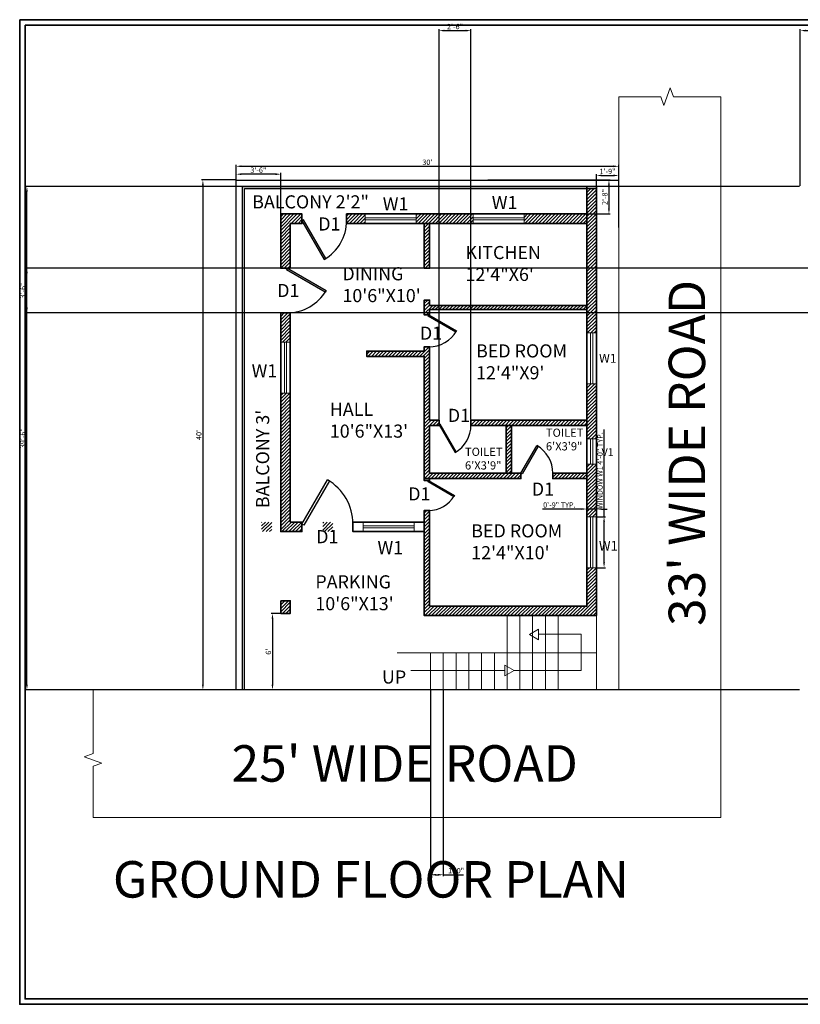
# Model space of a CAD drawing. Units: inches. Extents: x 2257 to 3849, y 1105 to 2032.
# Tile 1 of 2: x 2257 to 2992, y 1105 to 2032. Entities that reach past the tile are written whole.
import ezdxf

# ---------------------------------------------------------------- set-up
doc = ezdxf.new("R2010")
doc.units = ezdxf.units.IN
for name, color, linetype, lineweight in [('A-ANNO-DIMS', 7, 'Continuous', 18), ('A-ANNO-SYMB', 7, 'Continuous', 18), ('A-ANNO-TEXT', 130, 'Continuous', 18), ('A-ANNO-TTLB', 7, 'Continuous', 35), ('A-AREA-IDEN', 130, 'Continuous', 18), ('A-COLS', 10, 'Continuous', 35), ('A-FLOR-OTLN', 7, 'Continuous', 25), ('C-PROP', 7, 'Continuous', 25), ('C-ROAD', 7, 'Continuous', 18), ('Doors', 100, 'Continuous', 25), ('steps', 220, 'Continuous', 18), ('walls', 10, 'Continuous', 35), ('windows', 160, 'Continuous', 18)]:
    doc.layers.add(name, color=color, linetype=linetype, lineweight=lineweight)
doc.layers.add('A-COLS-PATT', color=40, linetype='Continuous', lineweight=13, true_color=0xf8d731)
doc.layers.add('A-WALL-PATT', color=241, linetype='Continuous', lineweight=13, true_color=0xf7abae)
doc.styles.get("Standard").update_dxf_attribs({"font": 'arial.ttf'})
doc.dimstyles.new('ISO-25', dxfattribs={"dimtxt": 5, "dimasz": 5, "dimexe": 1.25, "dimexo": 0.625, "dimtad": 1, "dimlunit": 3, "dimtxsty": 'Standard', "dimcen": 2.5, "dimadec": 0, "dimazin": 0, "dimtfac": 1, "dimtmove": 0, "dimatfit": 3, "dimfxl": 1, "dimarcsym": 0})

# ---------------------------------------------------------------- blocks, each defined once
blk = doc.blocks.new('*U4')
for p, q in [((0, 0), (0, -6)), ((40, 0), (40, -6))]:
    blk.add_line(p, q)
blk.add_lwpolyline([(0, 0), (20, 34.64), (21.52, 33.77), (1.52, -0.88)], close=True)
blk.add_arc((0, 0), 40, 0, 60)
blk = doc.blocks.new('*U5')
for p, q in [((-40, 0), (-40, 6)), ((0, 0), (0, 6))]:
    blk.add_line(p, q)
blk.add_lwpolyline([(0, 0), (-20, -34.64), (-21.52, -33.77), (-1.52, 0.87)], close=True)
blk.add_arc((0, 0), 40, 180, 240)
blk = doc.blocks.new('*U6')
for p, q in [((0, 0), (0, -6)), ((-40, 0), (-40, -6))]:
    blk.add_line(p, q)
blk.add_lwpolyline([(0, 0), (-20, 34.64), (-21.52, 33.77), (-1.52, -0.88)], close=True)
blk.add_arc((0, 0), 40, 120, 180)
blk = doc.blocks.new('*U7')
for p, q in [((-40, 0), (-40, 6)), ((0, 0), (0, 6))]:
    blk.add_line(p, q)
blk.add_lwpolyline([(0, 0), (-20, -34.6), (-21.5, -33.8), (-1.5, 0.9)], close=True)
blk.add_arc((0, 0), 40, 180, 240)
blk = doc.blocks.new('*D9')
at = {"layer": 'A-ANNO-DIMS', "color": 0, "lineweight": -2, "transparency": 16777216}
for p, q in [((2460.94, 1881.97), (2460.94, 1895.49)), ((2465.94, 1894.24), (2815.94, 1894.24)), ((2820.94, 1881.97), (2820.94, 1895.49))]:
    blk.add_line(p, q, dxfattribs=at)
at = {"layer": 'A-ANNO-DIMS', "color": 0, "transparency": 16777216}
for points in [[(2465.94, 1895.08), (2465.94, 1893.41), (2460.94, 1894.24)], [(2815.94, 1895.08), (2815.94, 1893.41), (2820.94, 1894.24)]]:
    blk.add_solid(points, dxfattribs=at)
at = {"layer": 'DEFPOINTS', "color": 0, "transparency": 16777216}
for p in [(2820.94, 1894.24), (2460.94, 1881.35), (2820.94, 1881.35)]:
    blk.add_point(p, dxfattribs=at)
at = {"layer": 'A-ANNO-DIMS', "color": 0, "transparency": 16777216, "insert": (2640.94, 1897.42), "char_height": 5, "attachment_point": 5}
blk.add_mtext("30'", dxfattribs=at)
blk = doc.blocks.new('*D10')
at = {"layer": 'A-ANNO-DIMS', "color": 0, "lineweight": -2, "transparency": 16777216}
for p, q in [((2460.32, 1881.35), (2428.52, 1881.35)), ((2429.77, 1876.35), (2429.77, 1406.35)), ((2460.32, 1401.35), (2428.52, 1401.35))]:
    blk.add_line(p, q, dxfattribs=at)
at = {"layer": 'A-ANNO-DIMS', "color": 0, "transparency": 16777216}
for points in [[(2428.94, 1876.35), (2430.61, 1876.35), (2429.77, 1881.35)], [(2428.94, 1406.35), (2430.61, 1406.35), (2429.77, 1401.35)]]:
    blk.add_solid(points, dxfattribs=at)
at = {"layer": 'DEFPOINTS', "color": 0, "transparency": 16777216}
for p in [(2460.94, 1881.35), (2429.77, 1401.35), (2460.94, 1401.35)]:
    blk.add_point(p, dxfattribs=at)
at = {"layer": 'A-ANNO-DIMS', "color": 0, "transparency": 16777216, "insert": (2426.6, 1641.35), "char_height": 5, "attachment_point": 5, "rotation": 90}
blk.add_mtext("40'", dxfattribs=at)
blk = doc.blocks.new('*D11')
at = {"layer": 'A-ANNO-DIMS', "color": 0, "lineweight": -2, "transparency": 16777216}
for p, q in [((2697.88, 1881.35), (2812.97, 1881.35)), ((2811.72, 1876.35), (2811.72, 1854.35)), ((2690.41, 1849.35), (2812.97, 1849.35))]:
    blk.add_line(p, q, dxfattribs=at)
at = {"layer": 'A-ANNO-DIMS', "color": 0, "transparency": 16777216}
for points in [[(2810.89, 1876.35), (2812.55, 1876.35), (2811.72, 1881.35)], [(2810.89, 1854.35), (2812.55, 1854.35), (2811.72, 1849.35)]]:
    blk.add_solid(points, dxfattribs=at)
at = {"layer": 'DEFPOINTS', "color": 0, "transparency": 16777216}
for p in [(2697.25, 1881.35), (2689.78, 1849.35), (2811.72, 1849.35)]:
    blk.add_point(p, dxfattribs=at)
at = {"layer": 'A-ANNO-DIMS', "color": 0, "transparency": 16777216, "insert": (2808.54, 1865.35), "char_height": 5, "attachment_point": 5, "rotation": 90}
blk.add_mtext('2\'-8"', dxfattribs=at)
blk = doc.blocks.new('*D12')
at = {"layer": 'A-ANNO-DIMS', "color": 0, "lineweight": -2, "transparency": 16777216}
for p, q in [((2460.94, 1824.47), (2460.94, 1888.06)), ((2497.94, 1886.81), (2465.94, 1886.81)), ((2502.94, 1824.47), (2502.94, 1888.06))]:
    blk.add_line(p, q, dxfattribs=at)
at = {"layer": 'A-ANNO-DIMS', "color": 0, "transparency": 16777216}
for points in [[(2465.94, 1887.65), (2465.94, 1885.98), (2460.94, 1886.81)], [(2497.94, 1887.65), (2497.94, 1885.98), (2502.94, 1886.81)]]:
    blk.add_solid(points, dxfattribs=at)
at = {"layer": 'DEFPOINTS', "color": 0, "transparency": 16777216}
for p in [(2460.94, 1886.81), (2460.94, 1823.85), (2502.94, 1823.85)]:
    blk.add_point(p, dxfattribs=at)
at = {"layer": 'A-ANNO-DIMS', "color": 0, "transparency": 16777216, "insert": (2481.94, 1889.99), "char_height": 5, "attachment_point": 5}
blk.add_mtext('3\'-6"', dxfattribs=at)
blk = doc.blocks.new('*D13')
at = {"layer": 'A-ANNO-DIMS', "color": 0, "lineweight": -2, "transparency": 16777216}
for p, q in [((2799.94, 1836.7), (2799.94, 1886.87)), ((2804.94, 1885.62), (2815.94, 1885.62)), ((2820.94, 1836.7), (2820.94, 1886.87))]:
    blk.add_line(p, q, dxfattribs=at)
at = {"layer": 'A-ANNO-DIMS', "color": 0, "transparency": 16777216}
for points in [[(2804.94, 1886.45), (2804.94, 1884.78), (2799.94, 1885.62)], [(2815.94, 1886.45), (2815.94, 1884.78), (2820.94, 1885.62)]]:
    blk.add_solid(points, dxfattribs=at)
at = {"layer": 'DEFPOINTS', "color": 0, "transparency": 16777216}
for p in [(2820.94, 1885.62), (2799.94, 1836.07), (2820.94, 1836.07)]:
    blk.add_point(p, dxfattribs=at)
at = {"layer": 'A-ANNO-DIMS', "color": 0, "transparency": 16777216, "insert": (2810.44, 1888.8), "char_height": 5, "attachment_point": 5}
blk.add_mtext('1\'-9"', dxfattribs=at)
blk = doc.blocks.new('*D14')
at = {"layer": 'A-ANNO-DIMS', "color": 0, "lineweight": -2, "transparency": 16777216}
for p, q in [((2511.32, 1473.35), (2493.97, 1473.35)), ((2495.22, 1468.35), (2495.22, 1406.35)), ((2511.32, 1401.35), (2493.97, 1401.35))]:
    blk.add_line(p, q, dxfattribs=at)
at = {"layer": 'A-ANNO-DIMS', "color": 0, "transparency": 16777216}
for points in [[(2494.39, 1468.35), (2496.05, 1468.35), (2495.22, 1473.35)], [(2494.39, 1406.35), (2496.05, 1406.35), (2495.22, 1401.35)]]:
    blk.add_solid(points, dxfattribs=at)
at = {"layer": 'DEFPOINTS', "color": 0, "transparency": 16777216}
for p in [(2511.94, 1473.35), (2495.22, 1401.35), (2511.94, 1401.35)]:
    blk.add_point(p, dxfattribs=at)
at = {"layer": 'A-ANNO-DIMS', "color": 0, "transparency": 16777216, "insert": (2492.04, 1437.35), "char_height": 5, "attachment_point": 5, "rotation": 90}
blk.add_mtext("6'", dxfattribs=at)
blk = doc.blocks.new('WIN-W1-48IN')
for p, q in [((0, 5.5), (48, 5.5)), ((0, 3.5), (48, 3.5))]:
    blk.add_line(p, q)
blk.add_lwpolyline([(0, 9), (48, 9), (48, 0), (0, 0)], close=True)
blk = doc.blocks.new('VENT-V1-24IN')
for p, q in [((3.5, 0), (3.5, 24)), ((5.5, 0), (5.5, 24))]:
    blk.add_line(p, q)
blk.add_lwpolyline([(0, 0), (0, 24), (9, 24), (9, 0)], close=True)
blk = doc.blocks.new('STAIR-DIRECTION-RETURN')
for points in [[(96.97, 5.1), (160.01, 5.1), (160.01, 39.11), (120.14, 39.11)], [(0, 5.1), (88.35, 5.1)]]:
    blk.add_lwpolyline(points)
for points in [[(120.14, 34.02), (120.14, 44.09), (111.42, 39.05)], [(88.35, 10.07), (88.35, 0), (97.07, 5.03)]]:
    blk.add_lwpolyline(points, close=True)
blk = doc.blocks.new('*D18')
at = {"layer": 'A-ANNO-DIMS', "color": 0, "lineweight": -2, "transparency": 16777216}
for p, q in [((2807.14, 1564.44), (2807.14, 1646.38)), ((2800.57, 1564.44), (2808.39, 1564.44)), ((2807.14, 1521.44), (2807.14, 1559.44)), ((2800.57, 1516.44), (2808.39, 1516.44))]:
    blk.add_line(p, q, dxfattribs=at)
at = {"layer": 'A-ANNO-DIMS', "color": 0, "transparency": 16777216}
for points in [[(2806.31, 1559.44), (2807.98, 1559.44), (2807.14, 1564.44)], [(2806.31, 1521.44), (2807.98, 1521.44), (2807.14, 1516.44)]]:
    blk.add_solid(points, dxfattribs=at)
at = {"layer": 'DEFPOINTS', "color": 0, "transparency": 16777216}
for p in [(2799.94, 1564.44), (2807.14, 1564.44), (2799.94, 1516.44)]:
    blk.add_point(p, dxfattribs=at)
at = {"layer": 'A-ANNO-DIMS', "color": 0, "transparency": 16777216, "insert": (2803.93, 1607.91), "char_height": 5, "attachment_point": 5, "rotation": 90}
blk.add_mtext('WINDOW W1 4\'-0" TYP.', dxfattribs=at)
blk = doc.blocks.new('*D19')
at = {"layer": 'A-ANNO-DIMS', "color": 0, "lineweight": -2, "transparency": 16777216}
for p, q in [((2785.94, 1571.64), (2749.22, 1571.64)), ((2790.94, 1565.06), (2790.94, 1572.89)), ((2799.94, 1571.64), (2790.94, 1571.64)), ((2799.94, 1565.06), (2799.94, 1572.89)), ((2804.94, 1571.64), (2809.94, 1571.64))]:
    blk.add_line(p, q, dxfattribs=at)
at = {"layer": 'A-ANNO-DIMS', "color": 0, "transparency": 16777216}
for points in [[(2785.94, 1572.47), (2785.94, 1570.81), (2790.94, 1571.64)], [(2804.94, 1572.47), (2804.94, 1570.81), (2799.94, 1571.64)]]:
    blk.add_solid(points, dxfattribs=at)
at = {"layer": 'DEFPOINTS', "color": 0, "transparency": 16777216}
for p in [(2790.94, 1571.64), (2790.94, 1564.44), (2799.94, 1564.44)]:
    blk.add_point(p, dxfattribs=at)
at = {"layer": 'A-ANNO-DIMS', "color": 0, "transparency": 16777216, "insert": (2765.08, 1574.82), "char_height": 5, "attachment_point": 5}
blk.add_mtext('0\'-9" TYP.', dxfattribs=at)
blk = doc.blocks.new('*D22')
at = {"layer": 'A-ANNO-DIMS', "color": 0, "lineweight": -2, "transparency": 16777216}
for p, q in [((2991.73, 1875.97), (2991.73, 2023.22)), ((2996.73, 2021.97), (3319.73, 2021.97)), ((3324.73, 1875.97), (3324.73, 2023.22))]:
    blk.add_line(p, q, dxfattribs=at)
at = {"layer": 'A-ANNO-DIMS', "color": 0, "transparency": 16777216}
for points in [[(2996.73, 2022.81), (2996.73, 2021.14), (2991.73, 2021.97)], [(3319.73, 2022.81), (3319.73, 2021.14), (3324.73, 2021.97)]]:
    blk.add_solid(points, dxfattribs=at)
at = {"layer": 'DEFPOINTS', "color": 0, "transparency": 16777216}
for p in [(3324.73, 2021.97), (2991.73, 1875.35), (3324.73, 1875.35)]:
    blk.add_point(p, dxfattribs=at)
at = {"layer": 'A-ANNO-DIMS', "color": 0, "transparency": 16777216, "insert": (3158.23, 2025.15), "char_height": 5, "attachment_point": 5}
blk.add_mtext('27\'-9"', dxfattribs=at)
blk = doc.blocks.new('*D23')
at = {"layer": 'A-ANNO-DIMS', "color": 0, "lineweight": -2, "transparency": 16777216}
for p, q in [((2991.11, 1875.35), (2262.98, 1875.35)), ((2264.23, 1406.35), (2264.23, 1870.35)), ((2991.11, 1401.35), (2262.98, 1401.35))]:
    blk.add_line(p, q, dxfattribs=at)
at = {"layer": 'A-ANNO-DIMS', "color": 0, "transparency": 16777216}
for points in [[(2263.39, 1870.35), (2265.06, 1870.35), (2264.23, 1875.35)], [(2263.39, 1406.35), (2265.06, 1406.35), (2264.23, 1401.35)]]:
    blk.add_solid(points, dxfattribs=at)
at = {"layer": 'DEFPOINTS', "color": 0, "transparency": 16777216}
for p in [(2264.23, 1875.35), (2991.73, 1875.35), (2991.73, 1401.35)]:
    blk.add_point(p, dxfattribs=at)
at = {"layer": 'A-ANNO-DIMS', "color": 0, "transparency": 16777216, "insert": (2261.05, 1638.35), "char_height": 5, "attachment_point": 5, "rotation": 90}
blk.add_mtext('39\'-6"', dxfattribs=at)
blk = doc.blocks.new('*D25')
at = {"layer": 'A-ANNO-DIMS', "color": 0, "lineweight": -2, "transparency": 16777216}
for p, q in [((3027.11, 1798.35), (2262.98, 1798.35)), ((2264.23, 1761.35), (2264.23, 1793.35)), ((3027.11, 1756.35), (2262.98, 1756.35))]:
    blk.add_line(p, q, dxfattribs=at)
at = {"layer": 'A-ANNO-DIMS', "color": 0, "transparency": 16777216}
for points in [[(2263.39, 1793.35), (2265.06, 1793.35), (2264.23, 1798.35)], [(2263.39, 1761.35), (2265.06, 1761.35), (2264.23, 1756.35)]]:
    blk.add_solid(points, dxfattribs=at)
at = {"layer": 'DEFPOINTS', "color": 0, "transparency": 16777216}
for p in [(2264.23, 1798.35), (3027.73, 1798.35), (3027.73, 1756.35)]:
    blk.add_point(p, dxfattribs=at)
at = {"layer": 'A-ANNO-DIMS', "color": 0, "transparency": 16777216, "insert": (2261.05, 1777.35), "char_height": 5, "attachment_point": 5, "rotation": 90}
blk.add_mtext('3\'-6"', dxfattribs=at)
blk = doc.blocks.new('*D26')
at = {"layer": 'A-ANNO-DIMS', "color": 0, "lineweight": -2, "transparency": 16777216}
for p, q in [((2651.94, 1655.97), (2651.94, 2023.22)), ((2656.94, 2021.97), (2676.94, 2021.97)), ((2681.94, 1655.97), (2681.94, 2023.22))]:
    blk.add_line(p, q, dxfattribs=at)
at = {"layer": 'A-ANNO-DIMS', "color": 0, "transparency": 16777216}
for points in [[(2656.94, 2022.81), (2656.94, 2021.14), (2651.94, 2021.97)], [(2676.94, 2022.81), (2676.94, 2021.14), (2681.94, 2021.97)]]:
    blk.add_solid(points, dxfattribs=at)
at = {"layer": 'DEFPOINTS', "color": 0, "transparency": 16777216}
for p in [(2681.94, 2021.97), (2651.94, 1655.35), (2681.94, 1655.35)]:
    blk.add_point(p, dxfattribs=at)
at = {"layer": 'A-ANNO-DIMS', "color": 0, "transparency": 16777216, "insert": (2666.94, 2025.15), "char_height": 5, "attachment_point": 5}
blk.add_mtext('2\'-6"', dxfattribs=at)
blk = doc.blocks.new('*D27')
at = {"layer": 'A-ANNO-DIMS', "color": 0, "lineweight": -2, "transparency": 16777216}
for p, q in [((2643.94, 1400.72), (2643.94, 1226.15)), ((2655.94, 1400.72), (2655.94, 1226.15)), ((2648.94, 1227.4), (2650.94, 1227.4)), ((2655.94, 1227.4), (2675.01, 1227.4))]:
    blk.add_line(p, q, dxfattribs=at)
at = {"layer": 'A-ANNO-DIMS', "color": 0, "transparency": 16777216}
for points in [[(2648.94, 1228.23), (2648.94, 1226.56), (2643.94, 1227.4)], [(2650.94, 1228.23), (2650.94, 1226.56), (2655.94, 1227.4)]]:
    blk.add_solid(points, dxfattribs=at)
at = {"layer": 'DEFPOINTS', "color": 0, "transparency": 16777216}
for p in [(2643.94, 1401.35), (2655.94, 1401.35), (2655.94, 1227.4)]:
    blk.add_point(p, dxfattribs=at)
at = {"layer": 'A-ANNO-DIMS', "color": 0, "transparency": 16777216, "insert": (2667.98, 1230.57), "char_height": 5, "attachment_point": 5}
blk.add_mtext('1\'-0"', dxfattribs=at)

msp = doc.modelspace()

# ---------------------------------------------------------------- hatches: boundary and pattern name
at = {"layer": 'A-COLS-PATT'}
h = msp.add_hatch(dxfattribs=at)
h.set_pattern_fill('ANSI31', color=256, scale=0.72)
h.paths.add_polyline_path([(2511.943, 1485.347), (2502.943, 1485.347), (2502.943, 1473.347), (2511.943, 1473.347)])
at = {"layer": 'A-WALL-PATT'}
h = msp.add_hatch(dxfattribs=at)
h.set_pattern_fill('ANSI31', color=256, scale=0.72)
h.paths.add_polyline_path([(2511.943, 1840.347), (2522.943, 1840.347), (2522.943, 1849.347), (2502.943, 1849.347), (2502.943, 1798.347), (2511.943, 1798.347)])
h.paths.add_polyline_path([(2582.419, 1849.347), (2564.943, 1849.347), (2564.943, 1840.347), (2582.419, 1840.347)])
h.paths.add_polyline_path([(2790.943, 1849.347), (2732, 1849.347), (2732, 1840.347), (2790.943, 1840.347)])
h.paths.add_polyline_path([(2799.943, 1873.347), (2790.943, 1873.347), (2790.943, 1737.469), (2799.943, 1737.469)])
h.paths.add_polyline_path([(2511.943, 1756.347), (2502.943, 1756.347), (2502.943, 1728.812), (2511.943, 1728.812)])
h.paths.add_polyline_path([(2511.943, 1680.812), (2502.943, 1680.812), (2502.943, 1550.347), (2522.943, 1550.347), (2522.943, 1559.347), (2511.943, 1559.347)])
h = msp.add_hatch(dxfattribs=at)
h.set_pattern_fill('ANSI31', color=256, scale=0.72)
h.paths.add_polyline_path([(2684, 1849.347), (2630.419, 1849.347), (2630.419, 1840.347), (2684, 1840.347)])
h.paths.add_polyline_path([(2642.943, 1840.347), (2637.943, 1840.347), (2637.943, 1798.347), (2642.943, 1798.347)])
h.paths.add_polyline_path([(2790.943, 1763.347), (2642.943, 1763.347), (2642.943, 1768.347), (2637.943, 1768.347), (2637.943, 1754.347), (2642.943, 1754.347), (2642.943, 1759.347), (2790.943, 1759.347)])
h.paths.add_polyline_path([(2642.943, 1724.347), (2637.943, 1724.347), (2637.943, 1720.347), (2583.943, 1720.347), (2583.943, 1715.347), (2637.943, 1715.347), (2637.943, 1600.347), (2728.943, 1600.347), (2728.943, 1605.347), (2642.943, 1605.347), (2642.943, 1650.347), (2651.943, 1650.347), (2651.943, 1655.347), (2642.943, 1655.347)])
h.paths.add_polyline_path([(2790.943, 1655.347), (2681.943, 1655.347), (2681.943, 1650.347), (2790.943, 1650.347)])
h.paths.add_polyline_path([(2719.943, 1650.347), (2714.943, 1650.347), (2714.943, 1605.347), (2719.943, 1605.347)], flags=17)
h.paths.add_polyline_path([(2790.943, 1605.347), (2758.943, 1605.347), (2758.943, 1600.347), (2790.943, 1600.347)])
h.paths.add_polyline_path([(2799.943, 1689.469), (2790.943, 1689.469), (2790.943, 1637.826), (2799.943, 1637.826)])
h.paths.add_polyline_path([(2799.943, 1613.826), (2790.943, 1613.826), (2790.943, 1564.439), (2799.943, 1564.439)])
h.paths.add_polyline_path([(2799.943, 1516.439), (2790.943, 1516.439), (2790.943, 1480.347), (2642.943, 1480.347), (2642.943, 1570.347), (2637.943, 1570.347), (2637.943, 1471.347), (2799.943, 1471.347)])
h = msp.add_hatch(dxfattribs=at)
h.set_pattern_fill('ANSI31', color=256, scale=0.72)
h.set_pattern_definition([(45, (-85.9454, 0), (-1.6164461, 1.6164461), [])])
h.paths.add_polyline_path([(2551.998, 1559.347), (2542.498, 1559.347), (2542.498, 1550.347), (2551.998, 1550.347)])
h.paths.add_polyline_path([(2494.498, 1559.347), (2484.998, 1559.347), (2484.998, 1550.347), (2494.498, 1550.347)])
h.paths.add_polyline_path([(3036.731, 1680.812), (3027.731, 1680.812), (3027.731, 1471.347), (3047.694, 1471.347), (3047.694, 1478.53), (3047.731, 1480.347), (3036.731, 1480.347)])
h.paths.add_polyline_path([(3036.731, 1756.347), (3027.731, 1756.347), (3027.731, 1728.812), (3036.731, 1728.812)])

# ---------------------------------------------------------------- linework, layer by layer
at = {"layer": 'A-ANNO-SYMB'}
for points in [[(2820.943, 1959.78), (2860.449, 1959.78), (2863.449, 1951.537), (2869.449, 1968.022), (2872.449, 1959.78), (2916.943, 1959.78)], [(2326.421, 1401.347), (2326.421, 1341.54), (2318.178, 1338.54), (2334.663, 1332.54), (2326.421, 1329.54), (2326.421, 1281.347)]]:
    msp.add_lwpolyline(points, dxfattribs=at)
at = {"layer": 'A-ANNO-TTLB'}
for points in [[(2257.449, 2032.239), (3848.988, 2032.239), (3848.988, 1105.467), (2257.449, 1105.467)], [(2262.449, 2027.239), (3843.988, 2027.239), (3843.988, 1110.467), (2262.449, 1110.467)]]:
    msp.add_lwpolyline(points, close=True, dxfattribs=at)
at = {"layer": 'A-COLS'}
msp.add_line((2502.943, 1473.347), (2502.943, 1485.265), dxfattribs=at)
msp.add_lwpolyline([(2502.943, 1485.347), (2511.943, 1485.347), (2511.943, 1473.347), (2502.943, 1473.347)], close=True, dxfattribs=at)
at = {"layer": 'A-FLOR-OTLN'}
for p, q in [((2466.943, 1401.347), (2466.943, 1875.347)), ((2466.943, 1875.347), (2799.943, 1875.347))]:
    msp.add_line(p, q, dxfattribs=at)
msp.add_lwpolyline([(2468.943, 1401.347), (2468.943, 1873.347), (2799.943, 1873.347)], dxfattribs=at)
at = {"layer": 'C-PROP'}
for p, q in [((2460.943, 1401.347), (2460.943, 1881.347)), ((2460.943, 1881.347), (2820.943, 1881.347))]:
    msp.add_line(p, q, dxfattribs=at)
at = {"layer": 'C-ROAD'}
for p, q in [((2820.943, 1959.78), (2820.943, 1401.347)), ((2916.943, 1959.78), (2916.943, 1281.347)), ((2820.943, 1401.347), (2326.421, 1401.347)), ((2916.943, 1281.347), (2326.421, 1281.347))]:
    msp.add_line(p, q, dxfattribs=at)
at = {"layer": 'steps'}
for p, q in [((2715.943, 1471.347), (2715.943, 1401.347)), ((2739.943, 1471.347), (2739.943, 1401.347)), ((2751.943, 1471.347), (2751.943, 1401.347)), ((2763.943, 1471.347), (2763.943, 1401.347)), ((2799.943, 1471.347), (2799.943, 1401.347)), ((2612.501, 1436.347), (2799.943, 1436.347)), ((2643.943, 1436.347), (2643.943, 1401.347)), ((2655.943, 1436.347), (2655.943, 1401.347)), ((2667.943, 1436.347), (2667.943, 1401.347)), ((2679.943, 1436.347), (2679.943, 1401.347)), ((2691.943, 1436.347), (2691.943, 1401.347)), ((2703.943, 1436.347), (2703.943, 1401.347))]:
    msp.add_line(p, q, dxfattribs=at)
msp.add_lwpolyline([(2727.943, 1471.347), (2727.943, 1401.347)], close=True, dxfattribs=at)
at = {"layer": 'walls'}
for p, q in [((2799.943, 1875.347), (2799.943, 1471.347)), ((2714.943, 1650.347), (2714.943, 1605.347)), ((2719.943, 1650.347), (2719.943, 1605.347))]:
    msp.add_line(p, q, dxfattribs=at)
for points in [[(2799.943, 1471.347), (2637.943, 1471.347), (2637.943, 1570.347), (2642.943, 1570.347), (2642.943, 1480.347), (2790.943, 1480.347), (2790.943, 1875.347)], [(2790.943, 1840.347), (2564.943, 1840.347), (2564.943, 1849.347), (2790.943, 1849.347)], [(2642.943, 1840.347), (2642.943, 1798.347), (2637.943, 1798.347), (2637.943, 1840.347)], [(2790.943, 1759.347), (2642.943, 1759.347), (2642.943, 1754.347), (2637.943, 1754.347), (2637.943, 1768.347), (2642.943, 1768.347), (2642.943, 1763.347), (2790.943, 1763.347)], [(2790.943, 1655.347), (2681.943, 1655.347), (2681.943, 1650.347), (2790.943, 1650.347)], [(2790.943, 1605.347), (2758.943, 1605.347), (2758.943, 1600.347), (2790.943, 1600.347)], [(2637.943, 1550.347), (2570.943, 1550.347), (2570.943, 1559.347), (2637.943, 1559.347)]]:
    msp.add_lwpolyline(points, dxfattribs=at)
for points in [[(2511.943, 1798.347), (2511.943, 1840.347), (2522.943, 1840.347), (2522.943, 1849.347), (2502.943, 1849.347), (2502.943, 1798.347)], [(2511.943, 1559.347), (2511.943, 1756.347), (2502.943, 1756.347), (2502.943, 1550.347), (2522.943, 1550.347), (2522.943, 1559.347)], [(2637.943, 1720.347), (2637.943, 1724.347), (2642.943, 1724.347), (2642.943, 1655.347), (2651.943, 1655.347), (2651.943, 1650.347), (2642.943, 1650.347), (2642.943, 1605.347), (2728.943, 1605.347), (2728.943, 1600.347), (2637.943, 1600.347), (2637.943, 1598.347), (2642.943, 1598.347), (2642.943, 1600.347), (2637.943, 1600.347), (2637.943, 1715.347), (2583.943, 1715.347), (2583.943, 1720.347)]]:
    msp.add_lwpolyline(points, close=True, dxfattribs=at)

# ---------------------------------------------------------------- block references
at = {"layer": 'A-ANNO-SYMB'}
msp.add_blockref('STAIR-DIRECTION-RETURN', (2625.459, 1414.636), dxfattribs=at)
at = {"layer": 'Doors'}
for name, p, xscale, yscale, zscale, rotation in [('*U6', (2522.943, 1843.047), 1.049999999999999, 1.049999999999999, 1.049999999999999, 180), ('*U5', (2509.243, 1798.347), 1.049999999999999, 1.049999999999999, 1.049999999999999, 90), ('*U5', (2642.443, 1754.347), 0.75, 0.75, 0.75, 90), ('*U6', (2651.943, 1650.849), 0.7496246408594235, 0.7496246408594235, 0.7496246408594235, 180), ('*U7', (2728.943, 1605.347), 0.7496246408594235, 0.7496246408594235, 0.7496246408594235, 180), ('*U5', (2642.143, 1598.347), 0.6999999999999944, 0.6999999999999944, 0.6999999999999944, 90)]:
    msp.add_blockref(name, p, dxfattribs=dict(at, xscale=xscale, yscale=yscale, zscale=zscale, rotation=rotation))
at = {"layer": 'Doors', "xscale": 1.200942847219647, "yscale": 1.200942847219647, "zscale": 1.200942847219647}
msp.add_blockref('*U4', (2522.905, 1557.53), dxfattribs=at)
at = {"layer": 'windows'}
for name, p in [('WIN-W1-48IN', (2582.419, 1840.347)), ('WIN-W1-48IN', (2684, 1840.347)), ('VENT-V1-24IN', (2790.943, 1613.826)), ('WIN-W1-48IN', (2580.443, 1550.347))]:
    msp.add_blockref(name, p, dxfattribs=at)
for p, rotation in [((2799.943, 1689.469), 90.00000000000111), ((2511.943, 1680.812), 90.00000000000111), ((2799.943, 1516.439), 90.00000000000094)]:
    msp.add_blockref('WIN-W1-48IN', p, dxfattribs=dict(at, rotation=rotation))

# ---------------------------------------------------------------- texts
at = {"layer": 'A-ANNO-TEXT', "attachment_point": 1}
for s, width, gutter_width, insert, char_height in [('W1', 167.82029, 61.663, (2598.98, 1865.042), 12.3325), ('W1', 167.82029, 61.663, (2701.516, 1866.238), 12.3325), ('D1', 167.82029, 61.663, (2538.314, 1846.134), 12.3325), ('D1', 167.82029, 61.663, (2499.669, 1783.521), 12.3325), ('D1', 167.82029, 61.663, (2633.927, 1743.35), 12.3325), ('W1', 114.48409, 42.065, (2802.474, 1717.711), 8.413), ('W1', 167.82029, 61.663, (2475.613, 1707.912), 12.3325), ('D1', 167.82029, 61.663, (2660.159, 1665.964), 12.3325), ('V1', 100.10563, 36.782, (2804.811, 1628.888), 7.3564), ('D1', 167.82029, 61.663, (2739.174, 1596.568), 12.3325), ('D1', 167.82029, 61.663, (2622.916, 1592.042), 12.3325), ('D1', 167.82029, 61.663, (2536.351, 1551.812), 12.3325), ('W1', 167.82029, 61.663, (2594.022, 1541.459), 12.3325), ('W1', 124.29149, 45.669, (2802.302, 1541.615), 9.1337), ('UP', 167.82029, 61.663, (2598.243, 1419.732), 12.3325), ("25' WIDE ROAD", 467.04814, 171.608, (2456.715, 1349.349), 34.32167), ('GROUND FLOOR PLAN', 551.57297, 171.608, (2345.141, 1240.242), 34.32167)]:
    msp.add_mtext_dynamic_manual_height_columns(s, width=width, gutter_width=gutter_width, heights=[0], dxfattribs=dict(at, insert=insert, char_height=char_height))
at = {"layer": 'A-ANNO-TEXT', "insert": (2867.879, 1461.542), "char_height": 34.32167, "attachment_point": 1, "rotation": 90}
msp.add_mtext_dynamic_manual_height_columns("33' WIDE ROAD", width=467.04814, gutter_width=171.608, heights=[0], dxfattribs=at)
at = {"layer": 'A-AREA-IDEN', "attachment_point": 1}
for s, width, gutter_width, insert, char_height in [('BALCONY 2\'2"', 254.30567, 61.663, (2476.142, 1866.935), 12.3325), ('KITCHEN \\P12\'4"X6\'', 167.82029, 61.663, (2676.8, 1819.217), 12.3325), ('DINING \\P10\'6"X10\'', 167.82029, 61.663, (2561.021, 1799.256), 12.3325), ('BED ROOM\\P12\'4"X9\'', 167.82029, 61.663, (2686.73, 1726.65), 12.3325), ('HALL \\P10\'6"X13\'', 167.82029, 61.663, (2549.158, 1671.698), 12.3325), ('TOILET\\P6\'X3\'9"', 104.71521, 38.476, (2752.437, 1647.35), 7.6951), ('TOILET\\P6\'X3\'9"', 104.71521, 38.476, (2676.303, 1629.38), 7.6951), ('BED ROOM  \\P12\'4"X10\'', 167.82029, 61.663, (2682.199, 1557.279), 12.3325), ('PARKING\\P10\'6"X13\'', 167.82029, 61.663, (2535.569, 1509.288), 12.3325)]:
    msp.add_mtext_dynamic_manual_height_columns(s, width=width, gutter_width=gutter_width, heights=[0], dxfattribs=dict(at, insert=insert, char_height=char_height))
at = {"layer": 'A-AREA-IDEN', "insert": (2479.797, 1572.53), "char_height": 12.3325, "attachment_point": 1, "rotation": 90}
msp.add_mtext_dynamic_manual_height_columns("BALCONY 3'", width=254.30567, gutter_width=61.663, heights=[0], dxfattribs=at)

# ---------------------------------------------------------------- dimensions: what is measured, and where the dimension line sits
at = {"layer": 'A-ANNO-DIMS'}
for base, p1, p2, override, picture, middle in [((2681.943, 2021.972), (2651.943, 1655.347), (2681.943, 1655.347), {"dimdec": 1, "dimlfac": 1, "dimrnd": 0, "dimzin": 1, "dimdsep": 46, "dimlunit": 4, "dimfrac": 2}, '*D26', (2666.943, 2025.15)), ((3324.731, 2021.972), (2991.731, 1875.347), (3324.731, 1875.347), {"dimdec": 1, "dimlfac": 1, "dimrnd": 0, "dimzin": 1, "dimdsep": 46, "dimlunit": 4, "dimfrac": 2}, '*D22', (3158.231, 2025.15)), ((2820.943, 1894.243), (2460.943, 1881.347), (2820.943, 1881.347), {"dimclrd": 0, "dimclre": 0, "dimclrt": 0}, '*D9', (2640.943, 1897.423)), ((2460.943, 1886.812), (2502.943, 1823.847), (2460.943, 1823.847), {"dimclrd": 0, "dimclre": 0, "dimclrt": 0}, '*D12', (2481.943, 1889.991)), ((2820.943, 1885.618), (2799.943, 1836.071), (2820.943, 1836.071), {"dimclrd": 0, "dimclre": 0, "dimclrt": 0}, '*D13', (2810.443, 1888.796)), ((2655.943, 1227.397), (2643.943, 1401.347), (2655.943, 1401.347), {"dimdec": 1, "dimlfac": 1, "dimrnd": 0, "dimzin": 1, "dimdsep": 46, "dimlunit": 4, "dimfrac": 2}, '*D27', (2667.978, 1230.574))]:
    dim = msp.add_linear_dim(base=base, p1=p1, p2=p2, dimstyle='ISO-25', override=override, dxfattribs=at)
    dim.commit()
    dim.dimension.update_dxf_attribs({"geometry": picture, "text_midpoint": middle})
for base, p1, p2, override, picture, middle in [((2264.228, 1875.347), (2991.731, 1401.347), (2991.731, 1875.347), {"dimdec": 1, "dimlfac": 1, "dimrnd": 0, "dimzin": 1, "dimdsep": 46, "dimlunit": 4, "dimfrac": 2}, '*D23', (2261.049, 1638.347)), ((2429.775, 1401.347), (2460.943, 1881.347), (2460.943, 1401.347), {"dimclrd": 0, "dimclre": 0, "dimclrt": 0}, '*D10', (2426.597, 1641.347)), ((2811.721, 1849.347), (2697.252, 1881.347), (2689.783, 1849.347), {"dimclrd": 0, "dimclre": 0, "dimclrt": 0}, '*D11', (2808.543, 1865.347)), ((2264.228, 1798.347), (3027.731, 1756.347), (3027.731, 1798.347), {"dimdec": 1, "dimlfac": 1, "dimrnd": 0, "dimzin": 1, "dimdsep": 46, "dimlunit": 4, "dimfrac": 2}, '*D25', (2261.049, 1777.347)), ((2495.22, 1401.347), (2511.943, 1473.347), (2511.943, 1401.347), {"dimclrd": 0, "dimclre": 0, "dimclrt": 0}, '*D14', (2492.042, 1437.347))]:
    dim = msp.add_linear_dim(base=base, p1=p1, p2=p2, angle=90, dimstyle='ISO-25', override=override, dxfattribs=at)
    dim.commit()
    dim.dimension.update_dxf_attribs({"geometry": picture, "text_midpoint": middle})
for base, p1, p2, angle, text, picture, middle in [((2807.143, 1564.439), (2799.943, 1516.439), (2799.943, 1564.439), 90, 'WINDOW W1 <> TYP.', '*D18', (2803.931, 1607.909)), ((2790.943, 1571.639), (2799.943, 1564.439), (2790.943, 1564.439), 180, '<> TYP.', '*D19', (2765.079, 1574.817))]:
    dim = msp.add_linear_dim(base=base, p1=p1, p2=p2, angle=angle, text=text, dimstyle='ISO-25', override={"dimdec": 1, "dimlfac": 1, "dimrnd": 0, "dimzin": 1, "dimdsep": 46, "dimlunit": 4, "dimfrac": 2}, dxfattribs=at)
    dim.commit()
    dim.dimension.update_dxf_attribs({"geometry": picture, "text_midpoint": middle})

doc.saveas('drawing.dxf')
